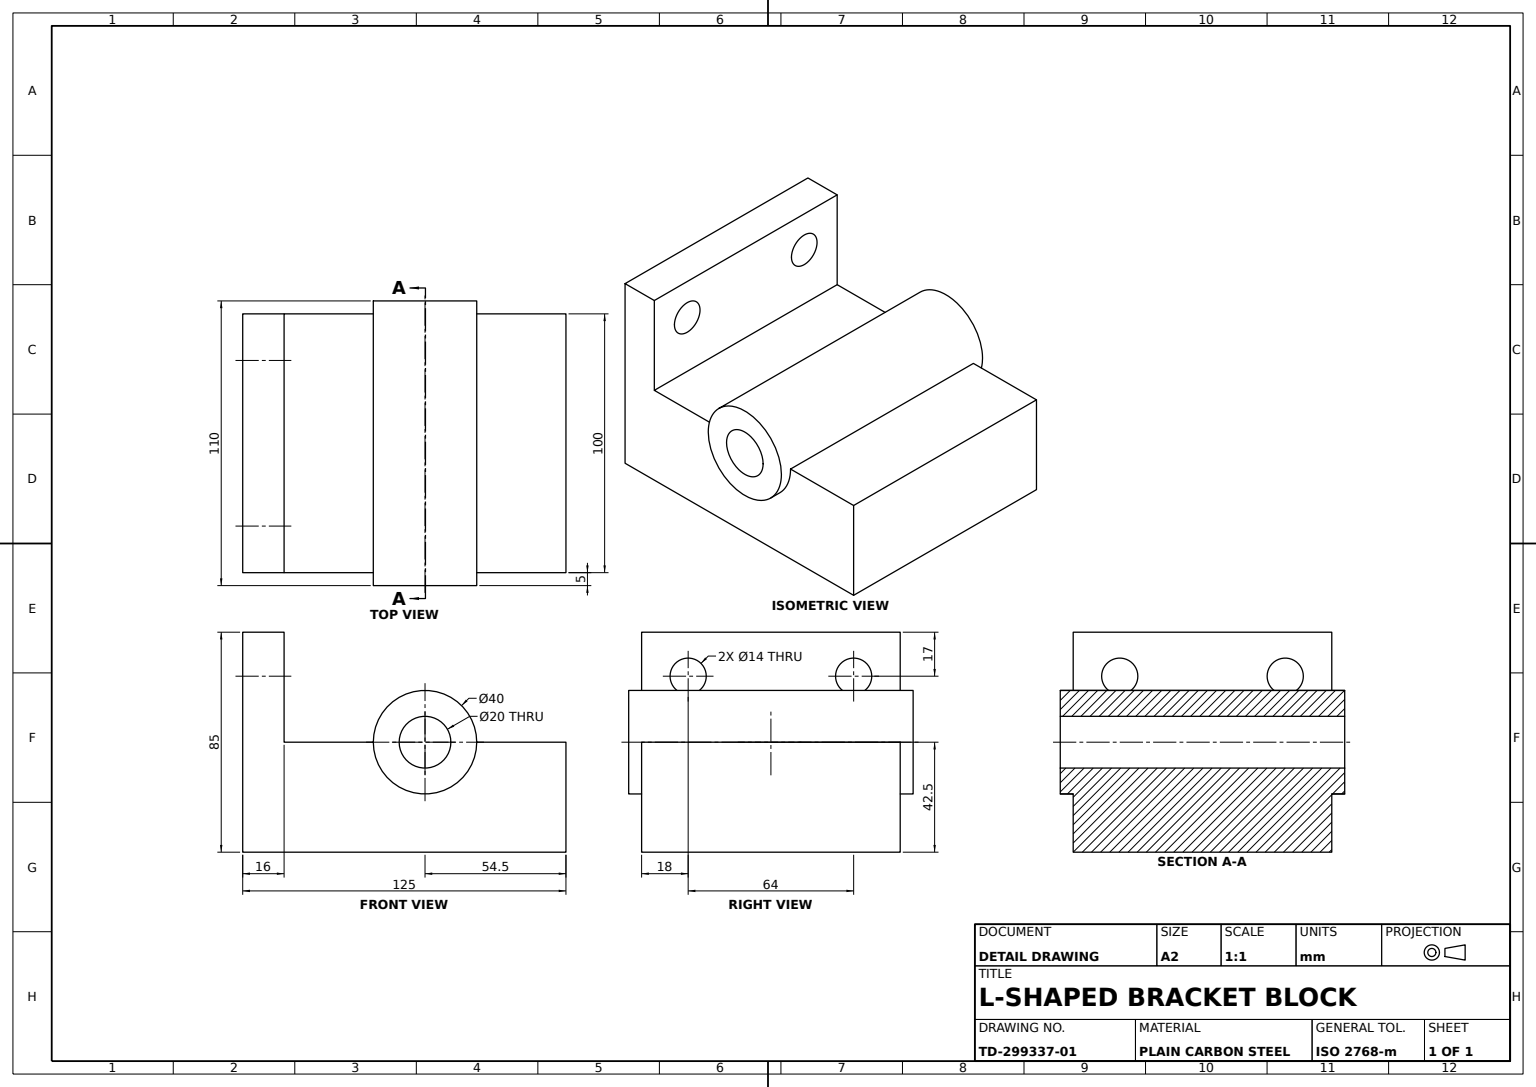
SolidWorks part; units mm, degrees
material "Plain Carbon Steel"
ref_plane "Front Plane" through (0, 0, 0) normal (0, 0, 1) x (1, 0, 0)
ref_plane "Top Plane" through (0, 0, 0) normal (0, 1, 0) x (1, 0, 0)
ref_plane "Right Plane" through (0, 0, 0) normal (1, 0, 0) x (0, 0, -1)
sketch "L Bracket Profile Sketch" plane through (0, 0, 0) normal (0, 0, 1) x (1, 0, 0)
  line L0 (0, 0) -> (125, 0)
  line L1 (125, 0) -> (125, 42.5)
  line L2 (0, 0) -> (0, 85)
  line L3 (0, 85) -> (16, 85)
  line L4 (16, 85) -> (16, 42.5)
  line L5 (125, 42.5) -> (16, 42.5)
  dimension "D1" = 125
  dimension "D2" = 42.5
  dimension "D3" = 85
  dimension "D4" = 16
extrude "L Bracket Body" add sketch "L Bracket Profile Sketch" against normal blind 100
sketch "Mounting Holes Sketch" plane through (16, 0, 0) normal (1, 0, 0) x (0, 0, -1)
  line L0 (100, 85) -> (0, 85) construction
  circle A0 centre (18, 68) radius 7
  circle A1 centre (82, 68) radius 7
  point P4 (50, 85)
  dimension "D1" = 14
  dimension "D4" = 14
  dimension "D2" = 17
  dimension "D3" = 32
  dimension "D5" = 17
  dimension "D6" = 32
extrude "Mounting Holes 2xØ14" cut sketch "Mounting Holes Sketch" against normal blind 100
sketch "Trunnion Sketch" plane through (0, 0, 0) normal (0, 0, 1) x (1, 0, 0)
  line L0 (125, 42.5) -> (16, 42.5) construction
  circle A0 centre (70.5, 42.5) radius 20
  dimension "D1" = 40
extrude "Trunnion Ø40" add sketch "Trunnion Sketch" against normal blind 100
sketch "Trunnion End Boss A Sketch" plane through (0, 0, 0) normal (0, 0, 1) x (1, 0, 0)
  circle A0 centre (70.5, 42.5) radius 20
  dimension "D1" = 40
extrude "Trunnion End Boss A Ø40x5" add sketch "Trunnion End Boss A Sketch" along normal blind 5
sketch "Trunnion End Boss B Sketch" plane through (0, 0, -100) normal (0, 0, -1) x (-1, 0, 0)
  circle A0 centre (-70.5, 42.5) radius 20
  dimension "D1" = 40
extrude "Trunnion End Boss B Ø40x5" add sketch "Trunnion End Boss B Sketch" along normal blind 5
sketch "Trunnion Bore Sketch" plane through (0, 0, -105) normal (0, 0, -1) x (-1, 0, 0)
  circle A0 centre (-70.5, 42.5) radius 10
  dimension "D1" = 20
extrude "Trunnion Bore Ø20" cut sketch "Trunnion Bore Sketch" against normal blind 110
